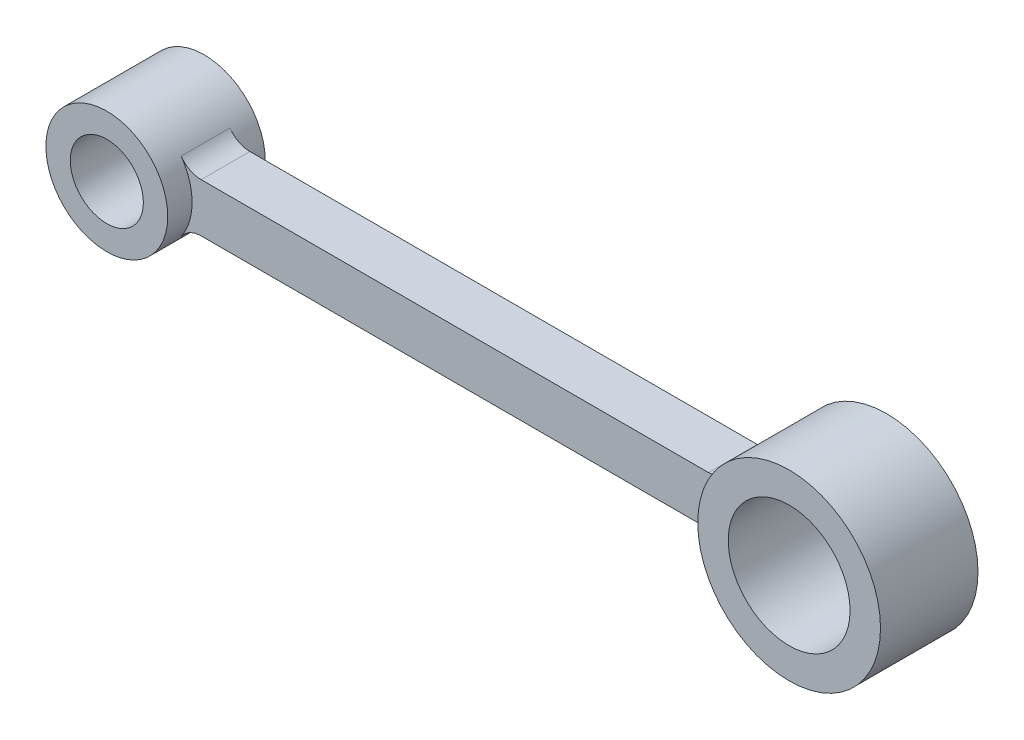
ISO-10303-21;
HEADER;
FILE_DESCRIPTION(('STEP AP214'),'2;1');
FILE_NAME('part.step','',(''),(''),'','','');
FILE_SCHEMA(('AUTOMOTIVE_DESIGN { 1 0 10303 214 1 1 1 1 }'));
ENDSEC;
DATA;
#1=APPLICATION_CONTEXT('core data for automotive mechanical design processes');
#2=APPLICATION_PROTOCOL_DEFINITION('international standard','automotive_design',2000,#1);
#3=PRODUCT_CONTEXT('',#1,'mechanical');
#4=PRODUCT('Part','Part','',(#3));
#5=PRODUCT_RELATED_PRODUCT_CATEGORY('part','',(#4));
#6=PRODUCT_DEFINITION_FORMATION('','',#4);
#7=PRODUCT_DEFINITION_CONTEXT('part definition',#1,'design');
#8=PRODUCT_DEFINITION('design','',#6,#7);
#9=PRODUCT_DEFINITION_SHAPE('','',#8);
#10=(LENGTH_UNIT() NAMED_UNIT(*) SI_UNIT(.MILLI.,.METRE.));
#11=(NAMED_UNIT(*) PLANE_ANGLE_UNIT() SI_UNIT($,.RADIAN.));
#12=(NAMED_UNIT(*) SI_UNIT($,.STERADIAN.) SOLID_ANGLE_UNIT());
#13=UNCERTAINTY_MEASURE_WITH_UNIT(LENGTH_MEASURE(1.E-05),#10,'distance_accuracy_value','');
#14=(GEOMETRIC_REPRESENTATION_CONTEXT(3) GLOBAL_UNCERTAINTY_ASSIGNED_CONTEXT((#13)) GLOBAL_UNIT_ASSIGNED_CONTEXT((#10,
#11,#12)) REPRESENTATION_CONTEXT('',''));
#15=CARTESIAN_POINT('',(0.,0.,0.));
#16=DIRECTION('',(0.,0.,1.));
#17=DIRECTION('',(1.,0.,0.));
#18=AXIS2_PLACEMENT_3D('',#15,#16,#17);
#19=CARTESIAN_POINT('',(-29.25,0.,4.));
#20=DIRECTION('',(0.,0.,1.));
#21=DIRECTION('',(1.,0.,0.));
#22=AXIS2_PLACEMENT_3D('',#19,#20,#21);
#23=PLANE('',#22);
#24=CARTESIAN_POINT('',(-29.25,0.,4.));
#25=DIRECTION('',(0.,0.,1.));
#26=DIRECTION('',(1.,0.,0.));
#27=AXIS2_PLACEMENT_3D('',#24,#25,#26);
#28=CIRCLE('',#27,5.);
#29=CARTESIAN_POINT('',(-24.25,0.,4.));
#30=VERTEX_POINT('',#29);
#31=EDGE_CURVE('E124',#30,#30,#28,.T.);
#32=ORIENTED_EDGE('',*,*,#31,.T.);
#33=EDGE_LOOP('',(#32));
#34=FACE_BOUND('',#33,.T.);
#35=CARTESIAN_POINT('',(-29.25,0.,4.));
#36=DIRECTION('',(0.,0.,1.));
#37=DIRECTION('',(1.,0.,0.));
#38=AXIS2_PLACEMENT_3D('',#35,#36,#37);
#39=CIRCLE('',#38,3.);
#40=CARTESIAN_POINT('',(-26.25,0.,4.));
#41=VERTEX_POINT('',#40);
#42=EDGE_CURVE('E185',#41,#41,#39,.T.);
#43=ORIENTED_EDGE('',*,*,#42,.F.);
#44=EDGE_LOOP('',(#43));
#45=FACE_BOUND('',#44,.T.);
#46=ADVANCED_FACE('F39',(#34,#45),#23,.T.);
#47=CARTESIAN_POINT('',(-29.25,0.,-4.));
#48=DIRECTION('',(0.,0.,1.));
#49=DIRECTION('',(1.,0.,0.));
#50=AXIS2_PLACEMENT_3D('',#47,#48,#49);
#51=PLANE('',#50);
#52=CARTESIAN_POINT('',(-29.25,0.,-4.));
#53=DIRECTION('',(0.,0.,1.));
#54=DIRECTION('',(1.,0.,0.));
#55=AXIS2_PLACEMENT_3D('',#52,#53,#54);
#56=CIRCLE('',#55,5.);
#57=CARTESIAN_POINT('',(-24.25,0.,-4.));
#58=VERTEX_POINT('',#57);
#59=EDGE_CURVE('E177',#58,#58,#56,.T.);
#60=ORIENTED_EDGE('',*,*,#59,.F.);
#61=EDGE_LOOP('',(#60));
#62=FACE_BOUND('',#61,.T.);
#63=CARTESIAN_POINT('',(-29.25,0.,-4.));
#64=DIRECTION('',(0.,0.,1.));
#65=DIRECTION('',(1.,0.,0.));
#66=AXIS2_PLACEMENT_3D('',#63,#64,#65);
#67=CIRCLE('',#66,3.);
#68=CARTESIAN_POINT('',(-26.25,0.,-4.));
#69=VERTEX_POINT('',#68);
#70=EDGE_CURVE('E183',#69,#69,#67,.T.);
#71=ORIENTED_EDGE('',*,*,#70,.T.);
#72=EDGE_LOOP('',(#71));
#73=FACE_BOUND('',#72,.T.);
#74=ADVANCED_FACE('F229',(#62,#73),#51,.F.);
#75=CARTESIAN_POINT('',(-29.25,0.,4.));
#76=DIRECTION('',(0.,0.,-1.));
#77=DIRECTION('',(-1.,0.,0.));
#78=AXIS2_PLACEMENT_3D('',#75,#76,#77);
#79=CYLINDRICAL_SURFACE('',#78,5.);
#80=CARTESIAN_POINT('',(-29.25,0.,-2.));
#81=DIRECTION('',(0.,0.,-1.));
#82=DIRECTION('',(1.,0.,0.));
#83=AXIS2_PLACEMENT_3D('',#80,#81,#82);
#84=CIRCLE('',#83,5.);
#85=CARTESIAN_POINT('',(-25.1467409667586,2.85714285714286,-2.));
#86=VERTEX_POINT('',#85);
#87=CARTESIAN_POINT('',(-25.1467409667586,-2.85714285714286,-2.));
#88=VERTEX_POINT('',#87);
#89=EDGE_CURVE('E53',#86,#88,#84,.T.);
#90=ORIENTED_EDGE('',*,*,#89,.T.);
#91=DIRECTION('',(0.,0.,-1.));
#92=VECTOR('',#91,1.);
#93=CARTESIAN_POINT('',(-25.1467409667586,-2.85714285714286,4.));
#94=LINE('',#93,#92);
#95=CARTESIAN_POINT('',(-25.1467409667586,-2.85714285714286,2.));
#96=VERTEX_POINT('',#95);
#97=EDGE_CURVE('E165',#88,#96,#94,.F.);
#98=ORIENTED_EDGE('',*,*,#97,.T.);
#99=CARTESIAN_POINT('',(-29.25,0.,2.));
#100=DIRECTION('',(0.,0.,-1.));
#101=DIRECTION('',(1.,0.,0.));
#102=AXIS2_PLACEMENT_3D('',#99,#100,#101);
#103=CIRCLE('',#102,5.);
#104=CARTESIAN_POINT('',(-25.1467409667586,2.85714285714286,2.));
#105=VERTEX_POINT('',#104);
#106=EDGE_CURVE('E63',#105,#96,#103,.T.);
#107=ORIENTED_EDGE('',*,*,#106,.F.);
#108=DIRECTION('',(0.,0.,-1.));
#109=VECTOR('',#108,1.);
#110=CARTESIAN_POINT('',(-25.1467409667586,2.85714285714286,4.));
#111=LINE('',#110,#109);
#112=EDGE_CURVE('E154',#105,#86,#111,.T.);
#113=ORIENTED_EDGE('',*,*,#112,.T.);
#114=EDGE_LOOP('',(#90,#98,#107,#113));
#115=FACE_BOUND('',#114,.T.);
#116=ORIENTED_EDGE('',*,*,#31,.F.);
#117=EDGE_LOOP('',(#116));
#118=FACE_BOUND('',#117,.T.);
#119=ORIENTED_EDGE('',*,*,#59,.T.);
#120=EDGE_LOOP('',(#119));
#121=FACE_BOUND('',#120,.T.);
#122=ADVANCED_FACE('F231',(#115,#118,#121),#79,.T.);
#123=CARTESIAN_POINT('',(-29.25,0.,4.));
#124=DIRECTION('',(0.,0.,-1.));
#125=DIRECTION('',(-1.,0.,0.));
#126=AXIS2_PLACEMENT_3D('',#123,#124,#125);
#127=CYLINDRICAL_SURFACE('',#126,3.);
#128=ORIENTED_EDGE('',*,*,#42,.T.);
#129=EDGE_LOOP('',(#128));
#130=FACE_BOUND('',#129,.T.);
#131=ORIENTED_EDGE('',*,*,#70,.F.);
#132=EDGE_LOOP('',(#131));
#133=FACE_BOUND('',#132,.T.);
#134=ADVANCED_FACE('F236',(#130,#133),#127,.F.);
#135=CARTESIAN_POINT('',(-24.6674243050442,2.,2.));
#136=DIRECTION('',(0.,-1.,0.));
#137=DIRECTION('',(0.,0.,-1.));
#138=AXIS2_PLACEMENT_3D('',#135,#136,#137);
#139=PLANE('',#138);
#140=DIRECTION('',(-1.,0.,0.));
#141=VECTOR('',#140,1.);
#142=CARTESIAN_POINT('',(-24.6674243050442,2.,2.));
#143=LINE('',#142,#141);
#144=CARTESIAN_POINT('',(18.1331560301929,2.,2.));
#145=VERTEX_POINT('',#144);
#146=CARTESIAN_POINT('',(-23.505437353462,2.,2.));
#147=VERTEX_POINT('',#146);
#148=EDGE_CURVE('E111',#145,#147,#143,.T.);
#149=ORIENTED_EDGE('',*,*,#148,.F.);
#150=DIRECTION('',(0.,0.,1.));
#151=VECTOR('',#150,1.);
#152=CARTESIAN_POINT('',(18.133156030193,2.,-2.));
#153=LINE('',#152,#151);
#154=CARTESIAN_POINT('',(18.1331560301929,2.,-2.));
#155=VERTEX_POINT('',#154);
#156=EDGE_CURVE('E128',#145,#155,#153,.F.);
#157=ORIENTED_EDGE('',*,*,#156,.T.);
#158=DIRECTION('',(-1.,0.,0.));
#159=VECTOR('',#158,1.);
#160=CARTESIAN_POINT('',(-24.6674243050442,2.,-2.));
#161=LINE('',#160,#159);
#162=CARTESIAN_POINT('',(-23.505437353462,2.,-2.));
#163=VERTEX_POINT('',#162);
#164=EDGE_CURVE('E145',#155,#163,#161,.T.);
#165=ORIENTED_EDGE('',*,*,#164,.T.);
#166=DIRECTION('',(0.,0.,1.));
#167=VECTOR('',#166,1.);
#168=CARTESIAN_POINT('',(-23.505437353462,2.,2.));
#169=LINE('',#168,#167);
#170=EDGE_CURVE('E147',#163,#147,#169,.T.);
#171=ORIENTED_EDGE('',*,*,#170,.T.);
#172=EDGE_LOOP('',(#149,#157,#165,#171));
#173=FACE_BOUND('',#172,.T.);
#174=ADVANCED_FACE('F149',(#173),#139,.F.);
#175=CARTESIAN_POINT('',(-24.6674243050442,-2.,2.));
#176=DIRECTION('',(0.,1.,0.));
#177=DIRECTION('',(0.,0.,1.));
#178=AXIS2_PLACEMENT_3D('',#175,#176,#177);
#179=PLANE('',#178);
#180=DIRECTION('',(1.,0.,0.));
#181=VECTOR('',#180,1.);
#182=CARTESIAN_POINT('',(-24.6674243050442,-2.,-2.));
#183=LINE('',#182,#181);
#184=CARTESIAN_POINT('',(-23.505437353462,-2.,-2.));
#185=VERTEX_POINT('',#184);
#186=CARTESIAN_POINT('',(18.1331560301929,-2.,-2.));
#187=VERTEX_POINT('',#186);
#188=EDGE_CURVE('E113',#185,#187,#183,.T.);
#189=ORIENTED_EDGE('',*,*,#188,.T.);
#190=DIRECTION('',(0.,0.,1.));
#191=VECTOR('',#190,1.);
#192=CARTESIAN_POINT('',(18.133156030193,-2.,2.));
#193=LINE('',#192,#191);
#194=CARTESIAN_POINT('',(18.1331560301929,-2.,2.));
#195=VERTEX_POINT('',#194);
#196=EDGE_CURVE('E153',#187,#195,#193,.T.);
#197=ORIENTED_EDGE('',*,*,#196,.T.);
#198=DIRECTION('',(1.,0.,0.));
#199=VECTOR('',#198,1.);
#200=CARTESIAN_POINT('',(-24.6674243050442,-2.,2.));
#201=LINE('',#200,#199);
#202=CARTESIAN_POINT('',(-23.505437353462,-2.,2.));
#203=VERTEX_POINT('',#202);
#204=EDGE_CURVE('E187',#203,#195,#201,.T.);
#205=ORIENTED_EDGE('',*,*,#204,.F.);
#206=DIRECTION('',(0.,0.,1.));
#207=VECTOR('',#206,1.);
#208=CARTESIAN_POINT('',(-23.505437353462,-2.,-2.));
#209=LINE('',#208,#207);
#210=EDGE_CURVE('E160',#203,#185,#209,.F.);
#211=ORIENTED_EDGE('',*,*,#210,.T.);
#212=EDGE_LOOP('',(#189,#197,#205,#211));
#213=FACE_BOUND('',#212,.T.);
#214=ADVANCED_FACE('F174',(#213),#179,.F.);
#215=CARTESIAN_POINT('',(26.75,0.,2.));
#216=DIRECTION('',(0.,0.,1.));
#217=DIRECTION('',(1.,0.,0.));
#218=AXIS2_PLACEMENT_3D('',#215,#216,#217);
#219=PLANE('',#218);
#220=CARTESIAN_POINT('',(26.75,0.,2.));
#221=DIRECTION('',(0.,0.,-1.));
#222=DIRECTION('',(1.,0.,0.));
#223=AXIS2_PLACEMENT_3D('',#220,#221,#222);
#224=CIRCLE('',#223,7.5);
#225=CARTESIAN_POINT('',(19.9472284448892,-3.1578947368421,2.));
#226=VERTEX_POINT('',#225);
#227=CARTESIAN_POINT('',(19.9472284448892,3.1578947368421,2.));
#228=VERTEX_POINT('',#227);
#229=EDGE_CURVE('E101',#226,#228,#224,.T.);
#230=ORIENTED_EDGE('',*,*,#229,.T.);
#231=CARTESIAN_POINT('',(18.133156030193,4.,2.));
#232=DIRECTION('',(0.,0.,1.));
#233=DIRECTION('',(1.,0.,0.));
#234=AXIS2_PLACEMENT_3D('',#231,#232,#233);
#235=CIRCLE('',#234,2.);
#236=EDGE_CURVE('E106',#228,#145,#235,.F.);
#237=ORIENTED_EDGE('',*,*,#236,.T.);
#238=ORIENTED_EDGE('',*,*,#148,.T.);
#239=CARTESIAN_POINT('',(-23.505437353462,4.,2.));
#240=DIRECTION('',(0.,0.,1.));
#241=DIRECTION('',(1.,0.,0.));
#242=AXIS2_PLACEMENT_3D('',#239,#240,#241);
#243=CIRCLE('',#242,2.);
#244=EDGE_CURVE('E11',#147,#105,#243,.F.);
#245=ORIENTED_EDGE('',*,*,#244,.T.);
#246=ORIENTED_EDGE('',*,*,#106,.T.);
#247=CARTESIAN_POINT('',(-23.505437353462,-4.,2.));
#248=DIRECTION('',(0.,0.,1.));
#249=DIRECTION('',(1.,0.,0.));
#250=AXIS2_PLACEMENT_3D('',#247,#248,#249);
#251=CIRCLE('',#250,2.);
#252=EDGE_CURVE('E135',#96,#203,#251,.F.);
#253=ORIENTED_EDGE('',*,*,#252,.T.);
#254=ORIENTED_EDGE('',*,*,#204,.T.);
#255=CARTESIAN_POINT('',(18.133156030193,-4.,2.));
#256=DIRECTION('',(0.,0.,1.));
#257=DIRECTION('',(1.,0.,0.));
#258=AXIS2_PLACEMENT_3D('',#255,#256,#257);
#259=CIRCLE('',#258,2.);
#260=EDGE_CURVE('E109',#195,#226,#259,.F.);
#261=ORIENTED_EDGE('',*,*,#260,.T.);
#262=EDGE_LOOP('',(#230,#237,#238,#245,#246,#253,#254,#261));
#263=FACE_BOUND('',#262,.T.);
#264=ADVANCED_FACE('F103',(#263),#219,.T.);
#265=CARTESIAN_POINT('',(26.75,0.,-2.));
#266=DIRECTION('',(0.,0.,1.));
#267=DIRECTION('',(1.,0.,0.));
#268=AXIS2_PLACEMENT_3D('',#265,#266,#267);
#269=PLANE('',#268);
#270=CARTESIAN_POINT('',(26.75,0.,-2.));
#271=DIRECTION('',(0.,0.,-1.));
#272=DIRECTION('',(1.,0.,0.));
#273=AXIS2_PLACEMENT_3D('',#270,#271,#272);
#274=CIRCLE('',#273,7.5);
#275=CARTESIAN_POINT('',(19.9472284448892,-3.1578947368421,-2.));
#276=VERTEX_POINT('',#275);
#277=CARTESIAN_POINT('',(19.9472284448892,3.1578947368421,-2.));
#278=VERTEX_POINT('',#277);
#279=EDGE_CURVE('E123',#276,#278,#274,.T.);
#280=ORIENTED_EDGE('',*,*,#279,.F.);
#281=CARTESIAN_POINT('',(18.133156030193,-4.,-2.));
#282=DIRECTION('',(0.,0.,1.));
#283=DIRECTION('',(1.,0.,0.));
#284=AXIS2_PLACEMENT_3D('',#281,#282,#283);
#285=CIRCLE('',#284,2.);
#286=EDGE_CURVE('E163',#276,#187,#285,.T.);
#287=ORIENTED_EDGE('',*,*,#286,.T.);
#288=ORIENTED_EDGE('',*,*,#188,.F.);
#289=CARTESIAN_POINT('',(-23.505437353462,-4.,-2.));
#290=DIRECTION('',(0.,0.,1.));
#291=DIRECTION('',(1.,0.,0.));
#292=AXIS2_PLACEMENT_3D('',#289,#290,#291);
#293=CIRCLE('',#292,2.);
#294=EDGE_CURVE('E133',#185,#88,#293,.T.);
#295=ORIENTED_EDGE('',*,*,#294,.T.);
#296=ORIENTED_EDGE('',*,*,#89,.F.);
#297=CARTESIAN_POINT('',(-23.505437353462,4.,-2.));
#298=DIRECTION('',(0.,0.,1.));
#299=DIRECTION('',(1.,0.,0.));
#300=AXIS2_PLACEMENT_3D('',#297,#298,#299);
#301=CIRCLE('',#300,2.);
#302=EDGE_CURVE('E50',#86,#163,#301,.T.);
#303=ORIENTED_EDGE('',*,*,#302,.T.);
#304=ORIENTED_EDGE('',*,*,#164,.F.);
#305=CARTESIAN_POINT('',(18.133156030193,4.,-2.));
#306=DIRECTION('',(0.,0.,1.));
#307=DIRECTION('',(1.,0.,0.));
#308=AXIS2_PLACEMENT_3D('',#305,#306,#307);
#309=CIRCLE('',#308,2.);
#310=EDGE_CURVE('E134',#155,#278,#309,.T.);
#311=ORIENTED_EDGE('',*,*,#310,.T.);
#312=EDGE_LOOP('',(#280,#287,#288,#295,#296,#303,#304,#311));
#313=FACE_BOUND('',#312,.T.);
#314=ADVANCED_FACE('F141',(#313),#269,.F.);
#315=CARTESIAN_POINT('',(26.75,0.,4.));
#316=DIRECTION('',(0.,0.,1.));
#317=DIRECTION('',(1.,0.,0.));
#318=AXIS2_PLACEMENT_3D('',#315,#316,#317);
#319=PLANE('',#318);
#320=CARTESIAN_POINT('',(26.75,0.,4.));
#321=DIRECTION('',(0.,0.,1.));
#322=DIRECTION('',(1.,0.,0.));
#323=AXIS2_PLACEMENT_3D('',#320,#321,#322);
#324=CIRCLE('',#323,7.5);
#325=CARTESIAN_POINT('',(34.25,0.,4.));
#326=VERTEX_POINT('',#325);
#327=EDGE_CURVE('E191',#326,#326,#324,.T.);
#328=ORIENTED_EDGE('',*,*,#327,.T.);
#329=EDGE_LOOP('',(#328));
#330=FACE_BOUND('',#329,.T.);
#331=CARTESIAN_POINT('',(26.75,0.,4.));
#332=DIRECTION('',(0.,0.,1.));
#333=DIRECTION('',(1.,0.,0.));
#334=AXIS2_PLACEMENT_3D('',#331,#332,#333);
#335=CIRCLE('',#334,5.);
#336=CARTESIAN_POINT('',(31.75,0.,4.));
#337=VERTEX_POINT('',#336);
#338=EDGE_CURVE('E199',#337,#337,#335,.T.);
#339=ORIENTED_EDGE('',*,*,#338,.F.);
#340=EDGE_LOOP('',(#339));
#341=FACE_BOUND('',#340,.T.);
#342=ADVANCED_FACE('F215',(#330,#341),#319,.T.);
#343=CARTESIAN_POINT('',(26.75,0.,-4.));
#344=DIRECTION('',(0.,0.,1.));
#345=DIRECTION('',(1.,0.,0.));
#346=AXIS2_PLACEMENT_3D('',#343,#344,#345);
#347=PLANE('',#346);
#348=CARTESIAN_POINT('',(26.75,0.,-4.));
#349=DIRECTION('',(0.,0.,1.));
#350=DIRECTION('',(1.,0.,0.));
#351=AXIS2_PLACEMENT_3D('',#348,#349,#350);
#352=CIRCLE('',#351,7.5);
#353=CARTESIAN_POINT('',(34.25,0.,-4.));
#354=VERTEX_POINT('',#353);
#355=EDGE_CURVE('E197',#354,#354,#352,.T.);
#356=ORIENTED_EDGE('',*,*,#355,.F.);
#357=EDGE_LOOP('',(#356));
#358=FACE_BOUND('',#357,.T.);
#359=CARTESIAN_POINT('',(26.75,0.,-4.));
#360=DIRECTION('',(0.,0.,1.));
#361=DIRECTION('',(1.,0.,0.));
#362=AXIS2_PLACEMENT_3D('',#359,#360,#361);
#363=CIRCLE('',#362,5.);
#364=CARTESIAN_POINT('',(31.75,0.,-4.));
#365=VERTEX_POINT('',#364);
#366=EDGE_CURVE('E201',#365,#365,#363,.T.);
#367=ORIENTED_EDGE('',*,*,#366,.T.);
#368=EDGE_LOOP('',(#367));
#369=FACE_BOUND('',#368,.T.);
#370=ADVANCED_FACE('F212',(#358,#369),#347,.F.);
#371=CARTESIAN_POINT('',(26.75,0.,4.));
#372=DIRECTION('',(0.,0.,-1.));
#373=DIRECTION('',(-1.,0.,0.));
#374=AXIS2_PLACEMENT_3D('',#371,#372,#373);
#375=CYLINDRICAL_SURFACE('',#374,7.5);
#376=DIRECTION('',(0.,0.,-1.));
#377=VECTOR('',#376,1.);
#378=CARTESIAN_POINT('',(19.9472284448892,-3.1578947368421,4.));
#379=LINE('',#378,#377);
#380=EDGE_CURVE('E122',#226,#276,#379,.T.);
#381=ORIENTED_EDGE('',*,*,#380,.T.);
#382=ORIENTED_EDGE('',*,*,#279,.T.);
#383=DIRECTION('',(0.,0.,-1.));
#384=VECTOR('',#383,1.);
#385=CARTESIAN_POINT('',(19.9472284448892,3.1578947368421,4.));
#386=LINE('',#385,#384);
#387=EDGE_CURVE('E117',#278,#228,#386,.F.);
#388=ORIENTED_EDGE('',*,*,#387,.T.);
#389=ORIENTED_EDGE('',*,*,#229,.F.);
#390=EDGE_LOOP('',(#381,#382,#388,#389));
#391=FACE_BOUND('',#390,.T.);
#392=ORIENTED_EDGE('',*,*,#327,.F.);
#393=EDGE_LOOP('',(#392));
#394=FACE_BOUND('',#393,.T.);
#395=ORIENTED_EDGE('',*,*,#355,.T.);
#396=EDGE_LOOP('',(#395));
#397=FACE_BOUND('',#396,.T.);
#398=ADVANCED_FACE('F120',(#391,#394,#397),#375,.T.);
#399=CARTESIAN_POINT('',(26.75,0.,4.));
#400=DIRECTION('',(0.,0.,-1.));
#401=DIRECTION('',(-1.,0.,0.));
#402=AXIS2_PLACEMENT_3D('',#399,#400,#401);
#403=CYLINDRICAL_SURFACE('',#402,5.);
#404=ORIENTED_EDGE('',*,*,#338,.T.);
#405=EDGE_LOOP('',(#404));
#406=FACE_BOUND('',#405,.T.);
#407=ORIENTED_EDGE('',*,*,#366,.F.);
#408=EDGE_LOOP('',(#407));
#409=FACE_BOUND('',#408,.T.);
#410=ADVANCED_FACE('F207',(#406,#409),#403,.F.);
#411=CARTESIAN_POINT('',(18.133156030193,-4.,4.));
#412=DIRECTION('',(0.,0.,-1.));
#413=DIRECTION('',(-1.,0.,0.));
#414=AXIS2_PLACEMENT_3D('',#411,#412,#413);
#415=CYLINDRICAL_SURFACE('',#414,2.);
#416=ORIENTED_EDGE('',*,*,#260,.F.);
#417=ORIENTED_EDGE('',*,*,#196,.F.);
#418=ORIENTED_EDGE('',*,*,#286,.F.);
#419=ORIENTED_EDGE('',*,*,#380,.F.);
#420=EDGE_LOOP('',(#416,#417,#418,#419));
#421=FACE_BOUND('',#420,.T.);
#422=ADVANCED_FACE('F178',(#421),#415,.F.);
#423=CARTESIAN_POINT('',(18.133156030193,4.,4.));
#424=DIRECTION('',(0.,0.,-1.));
#425=DIRECTION('',(-1.,0.,0.));
#426=AXIS2_PLACEMENT_3D('',#423,#424,#425);
#427=CYLINDRICAL_SURFACE('',#426,2.);
#428=ORIENTED_EDGE('',*,*,#236,.F.);
#429=ORIENTED_EDGE('',*,*,#387,.F.);
#430=ORIENTED_EDGE('',*,*,#310,.F.);
#431=ORIENTED_EDGE('',*,*,#156,.F.);
#432=EDGE_LOOP('',(#428,#429,#430,#431));
#433=FACE_BOUND('',#432,.T.);
#434=ADVANCED_FACE('F126',(#433),#427,.F.);
#435=CARTESIAN_POINT('',(-23.505437353462,-4.,4.));
#436=DIRECTION('',(0.,0.,-1.));
#437=DIRECTION('',(-1.,0.,0.));
#438=AXIS2_PLACEMENT_3D('',#435,#436,#437);
#439=CYLINDRICAL_SURFACE('',#438,2.);
#440=ORIENTED_EDGE('',*,*,#252,.F.);
#441=ORIENTED_EDGE('',*,*,#97,.F.);
#442=ORIENTED_EDGE('',*,*,#294,.F.);
#443=ORIENTED_EDGE('',*,*,#210,.F.);
#444=EDGE_LOOP('',(#440,#441,#442,#443));
#445=FACE_BOUND('',#444,.T.);
#446=ADVANCED_FACE('F248',(#445),#439,.F.);
#447=CARTESIAN_POINT('',(-23.505437353462,4.,4.));
#448=DIRECTION('',(0.,0.,-1.));
#449=DIRECTION('',(-1.,0.,0.));
#450=AXIS2_PLACEMENT_3D('',#447,#448,#449);
#451=CYLINDRICAL_SURFACE('',#450,2.);
#452=ORIENTED_EDGE('',*,*,#244,.F.);
#453=ORIENTED_EDGE('',*,*,#170,.F.);
#454=ORIENTED_EDGE('',*,*,#302,.F.);
#455=ORIENTED_EDGE('',*,*,#112,.F.);
#456=EDGE_LOOP('',(#452,#453,#454,#455));
#457=FACE_BOUND('',#456,.T.);
#458=ADVANCED_FACE('F41',(#457),#451,.F.);
#459=CLOSED_SHELL('',(#46,#74,#122,#134,#174,#214,#264,#314,#342,#370,#398,#410,#422,#434,#446,#458));
#460=MANIFOLD_SOLID_BREP('B2',#459);
#461=ADVANCED_BREP_SHAPE_REPRESENTATION('',(#18,#460),#14);
#462=SHAPE_DEFINITION_REPRESENTATION(#9,#461);
ENDSEC;
END-ISO-10303-21;
